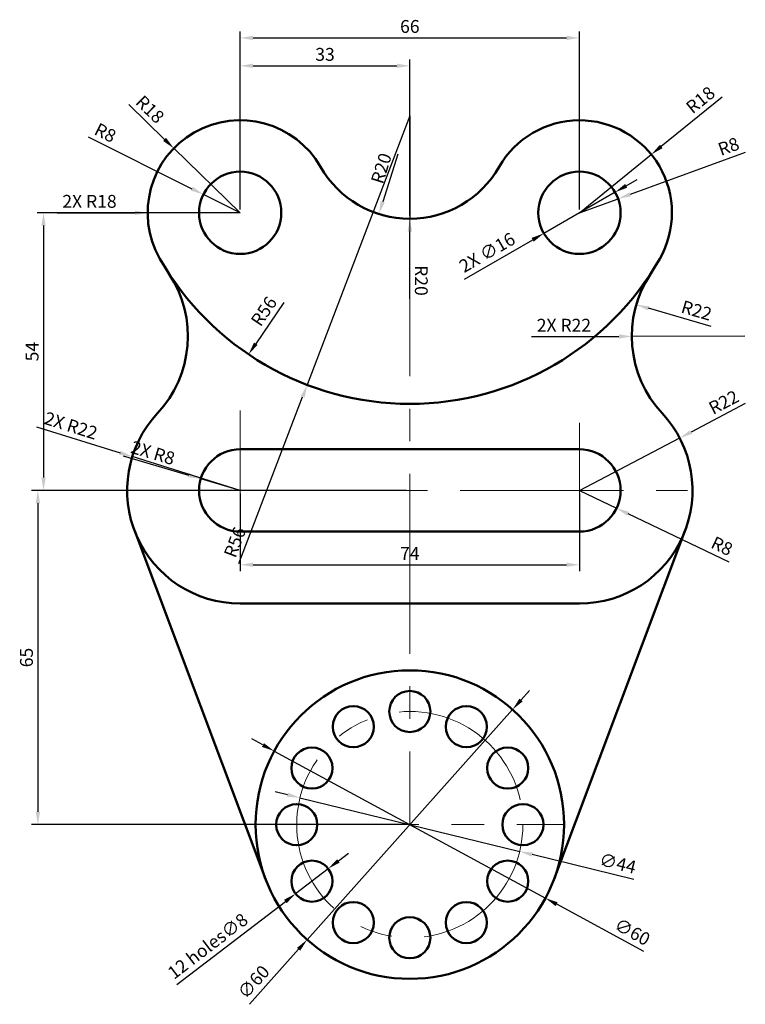
# Model space of a CAD drawing. Units: millimetres. Extents: x 2956 to 3097, y 1555 to 1747.
import ezdxf

# ---------------------------------------------------------------- set-up
doc = ezdxf.new("R2010")
doc.units = ezdxf.units.MM
doc.linetypes.add('CENTER', pattern=[50.8, 31.75, -6.35, 6.35, -6.35])
for name, color, linetype, lineweight in [('M-CNTR', 4, 'CENTER', 18), ('M-DIMS', 2, 'Continuous', 25), ('M-OUTL', 7, 'Continuous', 50)]:
    doc.layers.add(name, color=color, linetype=linetype, lineweight=lineweight)
doc.styles.get("Standard").update_dxf_attribs({"font": 'arial.ttf'})
doc.dimstyles.new('ISO-25', dxfattribs={"dimtxt": 2.5, "dimasz": 2.5, "dimexe": 1.25, "dimexo": 0.625, "dimtad": 1, "dimtxsty": 'Standard', "dimcen": 2.5, "dimadec": 0, "dimazin": 0, "dimtfac": 1, "dimtmove": 0, "dimatfit": 3, "dimfxl": 1, "dimarcsym": 0})

# ---------------------------------------------------------------- blocks, each defined once
blk = doc.blocks.new('*U2')
blk.add_circle((0, 0), 4)
blk = doc.blocks.new('*U3')
at = {"layer": 'M-OUTL', "color": 0, "linetype": 'ByBlock', "lineweight": -2, "transparency": 16777216}
for p, rotation in [((3020.97, 1609.09), 30), ((3042.97, 1609.09), 330), ((3012.92, 1601.04), 59.99999999999999), ((3051.02, 1601.04), 300), ((3009.97, 1590.04), 90), ((3053.97, 1590.04), 269.9999999999999), ((3012.92, 1579.04), 120), ((3051.02, 1579.04), 240), ((3020.97, 1570.99), 150), ((3042.97, 1570.99), 210), ((3031.97, 1568.04), 180)]:
    blk.add_blockref('*U2', p, dxfattribs=dict(at, rotation=rotation))
blk.add_blockref('*U2', (3031.97, 1612.04), dxfattribs=at)
blk = doc.blocks.new('*D4')
at = {"layer": 'Defpoints', "color": 0, "lineweight": -3, "transparency": 16777216}
for p in [(3064.97, 1743.06), (2998.97, 1709.04), (3064.97, 1709.04)]:
    blk.add_point(p, dxfattribs=at)
at = {"layer": 'M-DIMS', "color": 0, "lineweight": -2, "transparency": 16777216}
for p, q in [((2998.97, 1709.67), (2998.97, 1744.31)), ((3001.47, 1743.06), (3062.47, 1743.06)), ((3064.97, 1709.67), (3064.97, 1744.31))]:
    blk.add_line(p, q, dxfattribs=at)
at = {"layer": 'M-DIMS', "color": 0, "lineweight": -3, "transparency": 16777216}
for points in [[(3001.47, 1743.47), (3001.47, 1742.64), (2998.97, 1743.06)], [(3062.47, 1743.47), (3062.47, 1742.64), (3064.97, 1743.06)]]:
    blk.add_solid(points, dxfattribs=at)
at = {"layer": 'M-DIMS', "color": 0, "transparency": 16777216, "insert": (3031.97, 1744.96), "char_height": 2.5, "attachment_point": 5}
blk.add_mtext('66', dxfattribs=at)
blk = doc.blocks.new('*D5')
at = {"layer": 'Defpoints', "color": 0, "lineweight": -3, "transparency": 16777216}
for p in [(3078.95, 1720.38), (3064.97, 1709.04)]:
    blk.add_point(p, dxfattribs=at)
at = {"layer": 'M-DIMS', "color": 0, "lineweight": -2, "transparency": 16777216}
for p, q in [((3092.72, 1731.55), (3080.89, 1721.96)), ((3064.97, 1709.04), (3078.95, 1720.38))]:
    blk.add_line(p, q, dxfattribs=at)
at = {"layer": 'M-DIMS', "color": 0, "lineweight": -3, "transparency": 16777216}
blk.add_solid([(3080.63, 1722.28), (3081.15, 1721.63), (3078.95, 1720.38)], dxfattribs=at)
at = {"layer": 'M-DIMS', "color": 0, "transparency": 16777216, "insert": (3088.71, 1730.75), "char_height": 2.5, "attachment_point": 5, "rotation": 39.0521}
blk.add_mtext('R18', dxfattribs=at)
blk = doc.blocks.new('*D6')
at = {"layer": 'Defpoints', "color": 0, "lineweight": -3, "transparency": 16777216}
for p in [(3072.49, 1711.77), (3064.97, 1709.04)]:
    blk.add_point(p, dxfattribs=at)
at = {"layer": 'M-DIMS', "color": 0, "lineweight": -2, "transparency": 16777216}
for p, q in [((3097.22, 1720.76), (3074.84, 1712.63)), ((3064.97, 1709.04), (3072.49, 1711.77))]:
    blk.add_line(p, q, dxfattribs=at)
at = {"layer": 'M-DIMS', "color": 0, "lineweight": -3, "transparency": 16777216}
blk.add_solid([(3074.7, 1713.02), (3074.98, 1712.24), (3072.49, 1711.77)], dxfattribs=at)
at = {"layer": 'M-DIMS', "color": 0, "transparency": 16777216, "insert": (3094.09, 1721.65), "char_height": 2.5, "attachment_point": 5, "rotation": 19.9709}
blk.add_mtext('R8', dxfattribs=at)
blk = doc.blocks.new('*D7')
at = {"layer": 'Defpoints', "color": 0, "lineweight": -3, "transparency": 16777216}
for p in [(2991.81, 1712.61), (2998.97, 1709.04)]:
    blk.add_point(p, dxfattribs=at)
at = {"layer": 'M-DIMS', "color": 0, "lineweight": -2, "transparency": 16777216}
for p, q in [((2969.38, 1723.79), (2989.57, 1713.73)), ((2998.97, 1709.04), (2991.81, 1712.61))]:
    blk.add_line(p, q, dxfattribs=at)
at = {"layer": 'M-DIMS', "color": 0, "lineweight": -3, "transparency": 16777216}
blk.add_solid([(2989.76, 1714.1), (2989.39, 1713.35), (2991.81, 1712.61)], dxfattribs=at)
at = {"layer": 'M-DIMS', "color": 0, "transparency": 16777216, "insert": (2972.59, 1724.32), "char_height": 2.5, "attachment_point": 5, "rotation": 333.5006}
blk.add_mtext('R8', dxfattribs=at)
blk = doc.blocks.new('*D8')
at = {"layer": 'Defpoints', "color": 0, "lineweight": -3, "transparency": 16777216}
for p in [(2986.05, 1721.58), (2998.97, 1709.04)]:
    blk.add_point(p, dxfattribs=at)
at = {"layer": 'M-DIMS', "color": 0, "lineweight": -2, "transparency": 16777216}
for p, q in [((2977.28, 1730.09), (2984.26, 1723.32)), ((2998.97, 1709.04), (2986.05, 1721.58))]:
    blk.add_line(p, q, dxfattribs=at)
at = {"layer": 'M-DIMS', "color": 0, "lineweight": -3, "transparency": 16777216}
blk.add_solid([(2984.55, 1723.62), (2983.97, 1723.02), (2986.05, 1721.58)], dxfattribs=at)
at = {"layer": 'M-DIMS', "color": 0, "transparency": 16777216, "insert": (2981.2, 1728.94), "char_height": 2.5, "attachment_point": 5, "rotation": 315.858}
blk.add_mtext('R18', dxfattribs=at)
blk = doc.blocks.new('*D9')
at = {"layer": 'Defpoints', "color": 0, "lineweight": -3, "transparency": 16777216}
for p in [(2998.97, 1709.04), (2960.71, 1655.04), (2998.97, 1655.04)]:
    blk.add_point(p, dxfattribs=at)
at = {"layer": 'M-DIMS', "color": 0, "lineweight": -2, "transparency": 16777216}
for p, q in [((2998.34, 1709.04), (2959.46, 1709.04)), ((2960.71, 1706.54), (2960.71, 1657.54)), ((2998.34, 1655.04), (2959.46, 1655.04))]:
    blk.add_line(p, q, dxfattribs=at)
at = {"layer": 'M-DIMS', "color": 0, "lineweight": -3, "transparency": 16777216}
for points in [[(2960.29, 1706.54), (2961.12, 1706.54), (2960.71, 1709.04)], [(2960.29, 1657.54), (2961.12, 1657.54), (2960.71, 1655.04)]]:
    blk.add_solid(points, dxfattribs=at)
at = {"layer": 'M-DIMS', "color": 0, "transparency": 16777216, "insert": (2958.81, 1682.04), "char_height": 2.5, "attachment_point": 5, "rotation": 90}
blk.add_mtext('54', dxfattribs=at)
blk = doc.blocks.new('*D10')
at = {"layer": 'Defpoints', "color": 0, "lineweight": -3, "transparency": 16777216}
for p in [(3031.97, 1727.88), (3000.59, 1681.5)]:
    blk.add_point(p, dxfattribs=at)
at = {"layer": 'M-DIMS', "color": 0, "lineweight": -2, "transparency": 16777216}
blk.add_line((3007.44, 1691.62), (3001.99, 1683.57), dxfattribs=at)
at = {"layer": 'M-DIMS', "color": 0, "lineweight": -3, "transparency": 16777216}
blk.add_solid([(3001.65, 1683.8), (3002.34, 1683.34), (3000.59, 1681.5)], dxfattribs=at)
at = {"layer": 'M-DIMS', "color": 0, "transparency": 16777216, "insert": (3003.84, 1689.7), "char_height": 2.5, "attachment_point": 5, "rotation": 55.9212}
blk.add_mtext('R56', dxfattribs=at)
blk = doc.blocks.new('*D11')
at = {"layer": 'Defpoints', "color": 0, "lineweight": -3, "transparency": 16777216}
for p in [(3076.02, 1691.15), (3097.15, 1685.04)]:
    blk.add_point(p, dxfattribs=at)
at = {"layer": 'M-DIMS', "color": 0, "lineweight": -2, "transparency": 16777216}
blk.add_line((3090.61, 1686.93), (3078.42, 1690.46), dxfattribs=at)
at = {"layer": 'M-DIMS', "color": 0, "lineweight": -3, "transparency": 16777216}
blk.add_solid([(3078.54, 1690.86), (3078.3, 1690.06), (3076.02, 1691.15)], dxfattribs=at)
at = {"layer": 'M-DIMS', "color": 0, "transparency": 16777216, "insert": (3087.67, 1689.74), "char_height": 2.5, "attachment_point": 5, "rotation": 343.8873}
blk.add_mtext('R22', dxfattribs=at)
blk = doc.blocks.new('*D12')
at = {"layer": 'Defpoints', "color": 0, "lineweight": -3, "transparency": 16777216}
for p in [(3084.47, 1665.24), (3064.97, 1655.04)]:
    blk.add_point(p, dxfattribs=at)
at = {"layer": 'M-DIMS', "color": 0, "lineweight": -2, "transparency": 16777216}
for p, q in [((3097.24, 1671.92), (3086.68, 1666.39)), ((3064.97, 1655.04), (3084.47, 1665.24))]:
    blk.add_line(p, q, dxfattribs=at)
at = {"layer": 'M-DIMS', "color": 0, "lineweight": -3, "transparency": 16777216}
blk.add_solid([(3086.49, 1666.76), (3086.87, 1666.03), (3084.47, 1665.24)], dxfattribs=at)
at = {"layer": 'M-DIMS', "color": 0, "transparency": 16777216, "insert": (3093.18, 1671.91), "char_height": 2.5, "attachment_point": 5, "rotation": 27.6065}
blk.add_mtext('R22', dxfattribs=at)
blk = doc.blocks.new('*D13')
at = {"layer": 'Defpoints', "color": 0, "lineweight": -3, "transparency": 16777216}
for p in [(2998.97, 1655.04), (3064.97, 1655.04), (3064.97, 1640.58)]:
    blk.add_point(p, dxfattribs=at)
at = {"layer": 'M-DIMS', "color": 0, "lineweight": -2, "transparency": 16777216}
for p, q in [((2998.97, 1654.42), (2998.97, 1639.33)), ((3064.97, 1654.42), (3064.97, 1639.33)), ((3001.47, 1640.58), (3062.47, 1640.58))]:
    blk.add_line(p, q, dxfattribs=at)
at = {"layer": 'M-DIMS', "color": 0, "lineweight": -3, "transparency": 16777216}
for points in [[(3001.47, 1641), (3001.47, 1640.17), (2998.97, 1640.58)], [(3062.47, 1641), (3062.47, 1640.17), (3064.97, 1640.58)]]:
    blk.add_solid(points, dxfattribs=at)
at = {"layer": 'M-DIMS', "color": 0, "transparency": 16777216, "insert": (3031.97, 1642.46), "char_height": 2.5, "attachment_point": 5}
blk.add_mtext('74', dxfattribs=at)
blk = doc.blocks.new('*D14')
at = {"layer": 'Defpoints', "color": 0, "lineweight": -3, "transparency": 16777216}
for p in [(3064.97, 1655.04), (3072.18, 1651.59)]:
    blk.add_point(p, dxfattribs=at)
at = {"layer": 'M-DIMS', "color": 0, "lineweight": -2, "transparency": 16777216}
for p, q in [((3064.97, 1655.04), (3072.18, 1651.59)), ((3094.12, 1641.08), (3074.44, 1650.51))]:
    blk.add_line(p, q, dxfattribs=at)
at = {"layer": 'M-DIMS', "color": 0, "lineweight": -3, "transparency": 16777216}
blk.add_solid([(3074.62, 1650.88), (3074.26, 1650.13), (3072.18, 1651.59)], dxfattribs=at)
at = {"layer": 'M-DIMS', "color": 0, "transparency": 16777216, "insert": (3092.56, 1643.94), "char_height": 2.5, "attachment_point": 5, "rotation": 334.407}
blk.add_mtext('R8', dxfattribs=at)
blk = doc.blocks.new('*D15')
at = {"layer": 'Defpoints', "color": 0, "lineweight": -3, "transparency": 16777216}
for p in [(3031.97, 1655.04), (2959.61, 1590.04), (3031.97, 1590.04)]:
    blk.add_point(p, dxfattribs=at)
at = {"layer": 'M-DIMS', "color": 0, "lineweight": -2, "transparency": 16777216}
for p, q in [((3031.34, 1655.04), (2958.36, 1655.04)), ((2959.61, 1652.54), (2959.61, 1592.54)), ((3031.34, 1590.04), (2958.36, 1590.04))]:
    blk.add_line(p, q, dxfattribs=at)
at = {"layer": 'M-DIMS', "color": 0, "lineweight": -3, "transparency": 16777216}
for points in [[(2959.19, 1652.54), (2960.03, 1652.54), (2959.61, 1655.04)], [(2959.19, 1592.54), (2960.03, 1592.54), (2959.61, 1590.04)]]:
    blk.add_solid(points, dxfattribs=at)
at = {"layer": 'M-DIMS', "color": 0, "transparency": 16777216, "insert": (2957.71, 1622.54), "char_height": 2.5, "attachment_point": 5, "rotation": 90}
blk.add_mtext('65', dxfattribs=at)
blk = doc.blocks.new('*D16')
at = {"layer": 'Defpoints', "color": 0, "lineweight": -3, "transparency": 16777216}
for p in [(3031.97, 1727.88), (3025.95, 1708.81)]:
    blk.add_point(p, dxfattribs=at)
at = {"layer": 'M-DIMS', "color": 0, "lineweight": -2, "transparency": 16777216}
blk.add_line((3029.62, 1720.46), (3026.7, 1711.2), dxfattribs=at)
at = {"layer": 'M-DIMS', "color": 0, "lineweight": -3, "transparency": 16777216}
blk.add_solid([(3026.3, 1711.32), (3027.1, 1711.07), (3025.95, 1708.81)], dxfattribs=at)
at = {"layer": 'M-DIMS', "color": 0, "transparency": 16777216, "insert": (3026.72, 1717.59), "char_height": 2.5, "attachment_point": 5, "rotation": 72.4688}
blk.add_mtext('R20', dxfattribs=at)
blk = doc.blocks.new('*D17')
at = {"layer": 'Defpoints', "color": 0, "lineweight": -3, "transparency": 16777216}
for p in [(3010.6, 1595.26), (3053.34, 1584.82)]:
    blk.add_point(p, dxfattribs=at)
at = {"layer": 'M-DIMS', "color": 0, "lineweight": -2, "transparency": 16777216}
for p, q in [((3008.17, 1595.86), (3005.74, 1596.45)), ((3010.6, 1595.26), (3053.34, 1584.82)), ((3075.55, 1579.39), (3055.77, 1584.23))]:
    blk.add_line(p, q, dxfattribs=at)
at = {"layer": 'M-DIMS', "color": 0, "lineweight": -3, "transparency": 16777216}
for points in [[(3008.27, 1596.26), (3008.07, 1595.45), (3010.6, 1595.26)], [(3055.87, 1584.63), (3055.67, 1583.82), (3053.34, 1584.82)]]:
    blk.add_solid(points, dxfattribs=at)
at = {"layer": 'M-DIMS', "color": 0, "transparency": 16777216, "insert": (3072.35, 1582.2), "char_height": 2.5, "attachment_point": 5, "rotation": 346.271}
blk.add_mtext('∅44', dxfattribs=at)
blk = doc.blocks.new('*D18')
at = {"layer": 'Defpoints', "color": 0, "lineweight": -3, "transparency": 16777216}
for p in [(3051.95, 1612.42), (3011.99, 1567.66)]:
    blk.add_point(p, dxfattribs=at)
at = {"layer": 'M-DIMS', "color": 0, "lineweight": -2, "transparency": 16777216}
for p, q in [((3053.61, 1614.29), (3055.28, 1616.15)), ((3051.95, 1612.42), (3011.99, 1567.66)), ((3000.77, 1555.09), (3010.33, 1565.8))]:
    blk.add_line(p, q, dxfattribs=at)
at = {"layer": 'M-DIMS', "color": 0, "lineweight": -3, "transparency": 16777216}
for points in [[(3053.3, 1614.56), (3053.92, 1614.01), (3051.95, 1612.42)], [(3010.02, 1566.07), (3010.64, 1565.52), (3011.99, 1567.66)]]:
    blk.add_solid(points, dxfattribs=at)
at = {"layer": 'M-DIMS', "color": 0, "transparency": 16777216, "insert": (3001.81, 1559.22), "char_height": 2.5, "attachment_point": 5, "rotation": 48.2455}
blk.add_mtext('∅60', dxfattribs=at)
blk = doc.blocks.new('*D19')
at = {"layer": 'Defpoints', "color": 0, "lineweight": -3, "transparency": 16777216}
for p in [(3016.09, 1581.47), (3009.74, 1576.61)]:
    blk.add_point(p, dxfattribs=at)
at = {"layer": 'M-DIMS', "color": 0, "lineweight": -2, "transparency": 16777216}
for p, q in [((3018.08, 1582.99), (3020.06, 1584.51)), ((3016.09, 1581.47), (3009.74, 1576.61)), ((2986.67, 1558.95), (3007.76, 1575.09))]:
    blk.add_line(p, q, dxfattribs=at)
at = {"layer": 'M-DIMS', "color": 0, "lineweight": -3, "transparency": 16777216}
for points in [[(3017.83, 1583.32), (3018.33, 1582.66), (3016.09, 1581.47)], [(3007.5, 1575.42), (3008.01, 1574.76), (3009.74, 1576.61)]]:
    blk.add_solid(points, dxfattribs=at)
at = {"layer": 'M-DIMS', "color": 0, "transparency": 16777216, "insert": (2992.85, 1566.16), "char_height": 2.5, "attachment_point": 5, "rotation": 37.4262}
blk.add_mtext('12 holes∅8', dxfattribs=at)
blk = doc.blocks.new('HOLE-D16')
blk.add_circle((8, 8), 8)
blk = doc.blocks.new('*D21')
at = {"layer": 'Defpoints', "color": 0, "lineweight": -3, "transparency": 16777216}
for p in [(3031.97, 1737.63), (2998.97, 1709.04), (3031.97, 1707.88)]:
    blk.add_point(p, dxfattribs=at)
at = {"layer": 'M-DIMS', "color": 0, "lineweight": -2, "transparency": 16777216}
for p, q in [((2998.97, 1709.67), (2998.97, 1738.88)), ((3001.47, 1737.63), (3029.47, 1737.63)), ((3031.97, 1708.51), (3031.97, 1738.88))]:
    blk.add_line(p, q, dxfattribs=at)
at = {"layer": 'M-DIMS', "color": 0, "lineweight": -3, "transparency": 16777216}
for points in [[(3001.47, 1738.05), (3001.47, 1737.22), (2998.97, 1737.63)], [(3029.47, 1738.05), (3029.47, 1737.22), (3031.97, 1737.63)]]:
    blk.add_solid(points, dxfattribs=at)
at = {"layer": 'M-DIMS', "color": 0, "transparency": 16777216, "insert": (3015.47, 1739.53), "char_height": 2.5, "attachment_point": 5}
blk.add_mtext('33', dxfattribs=at)
blk = doc.blocks.new('*D22')
at = {"layer": 'Defpoints', "color": 0, "lineweight": -3, "transparency": 16777216}
for p in [(3071.9, 1713.04), (3058.04, 1705.04)]:
    blk.add_point(p, dxfattribs=at)
at = {"layer": 'M-DIMS', "color": 0, "lineweight": -2, "transparency": 16777216}
for p, q in [((3074.06, 1714.29), (3076.23, 1715.54)), ((3071.9, 1713.04), (3058.04, 1705.04)), ((3042.6, 1696.13), (3055.88, 1703.79))]:
    blk.add_line(p, q, dxfattribs=at)
at = {"layer": 'M-DIMS', "color": 0, "lineweight": -3, "transparency": 16777216}
for points in [[(3073.85, 1714.65), (3074.27, 1713.93), (3071.9, 1713.04)], [(3055.67, 1704.15), (3056.08, 1703.43), (3058.04, 1705.04)]]:
    blk.add_solid(points, dxfattribs=at)
at = {"layer": 'M-DIMS', "color": 0, "transparency": 16777216, "insert": (3047.17, 1701.04), "char_height": 2.5, "attachment_point": 5, "rotation": 30.0016}
blk.add_mtext('2X ∅16', dxfattribs=at)
blk = doc.blocks.new('*D23')
at = {"layer": 'Defpoints', "color": 0, "lineweight": -3, "transparency": 16777216}
for p in [(2980.97, 1709.04), (2998.97, 1709.04)]:
    blk.add_point(p, dxfattribs=at)
at = {"layer": 'M-DIMS', "color": 0, "lineweight": -2, "transparency": 16777216}
for p, q in [((2963.33, 1709.04), (2978.47, 1709.04)), ((2998.97, 1709.04), (2980.97, 1709.04))]:
    blk.add_line(p, q, dxfattribs=at)
at = {"layer": 'M-DIMS', "color": 0, "lineweight": -3, "transparency": 16777216}
blk.add_solid([(2978.47, 1709.46), (2978.47, 1708.62), (2980.97, 1709.04)], dxfattribs=at)
at = {"layer": 'M-DIMS', "color": 0, "transparency": 16777216, "insert": (2969.65, 1710.94), "char_height": 2.5, "attachment_point": 5, "rotation": 0.0005}
blk.add_mtext('2X R18', dxfattribs=at)
blk = doc.blocks.new('*D24')
at = {"layer": 'Defpoints', "color": 0, "lineweight": -3, "transparency": 16777216}
for p in [(3031.97, 1727.88), (3031.97, 1707.88)]:
    blk.add_point(p, dxfattribs=at)
at = {"layer": 'M-DIMS', "color": 0, "lineweight": -2, "transparency": 16777216}
for p, q in [((3031.97, 1727.88), (3031.97, 1707.88)), ((3031.97, 1692.28), (3031.97, 1705.38))]:
    blk.add_line(p, q, dxfattribs=at)
at = {"layer": 'M-DIMS', "color": 0, "lineweight": -3, "transparency": 16777216}
blk.add_solid([(3032.39, 1705.38), (3031.55, 1705.38), (3031.97, 1707.88)], dxfattribs=at)
at = {"layer": 'M-DIMS', "color": 0, "transparency": 16777216, "insert": (3033.87, 1695.88), "char_height": 2.5, "attachment_point": 5, "rotation": 270.0006}
blk.add_mtext('R20', dxfattribs=at)
blk = doc.blocks.new('*D25')
at = {"layer": 'Defpoints', "color": 0, "lineweight": -3, "transparency": 16777216}
for p in [(3031.97, 1727.88), (3012, 1675.56)]:
    blk.add_point(p, dxfattribs=at)
at = {"layer": 'M-DIMS', "color": 0, "lineweight": -2, "transparency": 16777216}
for p, q in [((3031.97, 1727.88), (3012, 1675.56)), ((2998.73, 1640.8), (3011.11, 1673.23))]:
    blk.add_line(p, q, dxfattribs=at)
at = {"layer": 'M-DIMS', "color": 0, "lineweight": -3, "transparency": 16777216}
blk.add_solid([(3010.72, 1673.38), (3011.5, 1673.08), (3012, 1675.56)], dxfattribs=at)
at = {"layer": 'M-DIMS', "color": 0, "transparency": 16777216, "insert": (2998.24, 1644.85), "char_height": 2.5, "attachment_point": 5, "rotation": 69.1098}
blk.add_mtext('R56', dxfattribs=at)
blk = doc.blocks.new('*D26')
at = {"layer": 'Defpoints', "color": 0, "lineweight": -3, "transparency": 16777216}
for p in [(3075.15, 1685), (3097.15, 1685.04)]:
    blk.add_point(p, dxfattribs=at)
at = {"layer": 'M-DIMS', "color": 0, "lineweight": -2, "transparency": 16777216}
for p, q in [((3055.65, 1684.96), (3072.65, 1685)), ((3097.15, 1685.04), (3075.15, 1685))]:
    blk.add_line(p, q, dxfattribs=at)
at = {"layer": 'M-DIMS', "color": 0, "lineweight": -3, "transparency": 16777216}
blk.add_solid([(3072.65, 1685.41), (3072.65, 1684.58), (3075.15, 1685)], dxfattribs=at)
at = {"layer": 'M-DIMS', "color": 0, "transparency": 16777216, "insert": (3061.95, 1686.85), "char_height": 2.5, "attachment_point": 5, "rotation": 0.1161}
blk.add_mtext('2X R22', dxfattribs=at)
blk = doc.blocks.new('*D27')
at = {"layer": 'Defpoints', "color": 0, "lineweight": -3, "transparency": 16777216}
for p in [(2977.97, 1661.61), (2998.97, 1655.04)]:
    blk.add_point(p, dxfattribs=at)
at = {"layer": 'M-DIMS', "color": 0, "lineweight": -2, "transparency": 16777216}
for p, q in [((2959.36, 1667.43), (2975.59, 1662.35)), ((2998.97, 1655.04), (2977.97, 1661.61))]:
    blk.add_line(p, q, dxfattribs=at)
at = {"layer": 'M-DIMS', "color": 0, "lineweight": -3, "transparency": 16777216}
blk.add_solid([(2975.71, 1662.75), (2975.46, 1661.96), (2977.97, 1661.61)], dxfattribs=at)
at = {"layer": 'M-DIMS', "color": 0, "transparency": 16777216, "insert": (2965.94, 1667.34), "char_height": 2.5, "attachment_point": 5, "rotation": 342.6316}
blk.add_mtext('2X R22', dxfattribs=at)
blk = doc.blocks.new('*D28')
at = {"layer": 'Defpoints', "color": 0, "lineweight": -3, "transparency": 16777216}
for p in [(2991.3, 1657.3), (2998.97, 1655.04)]:
    blk.add_point(p, dxfattribs=at)
at = {"layer": 'M-DIMS', "color": 0, "lineweight": -2, "transparency": 16777216}
for p, q in [((2976.23, 1661.74), (2988.9, 1658.01)), ((2998.97, 1655.04), (2991.3, 1657.3))]:
    blk.add_line(p, q, dxfattribs=at)
at = {"layer": 'M-DIMS', "color": 0, "lineweight": -3, "transparency": 16777216}
blk.add_solid([(2989.02, 1658.41), (2988.78, 1657.61), (2991.3, 1657.3)], dxfattribs=at)
at = {"layer": 'M-DIMS', "color": 0, "transparency": 16777216, "insert": (2981.9, 1662.05), "char_height": 2.5, "attachment_point": 5, "rotation": 343.5897}
blk.add_mtext('2X R8', dxfattribs=at)
blk = doc.blocks.new('*D29')
at = {"layer": 'Defpoints', "color": 0, "lineweight": -3, "transparency": 16777216}
for p in [(3005.59, 1604.34), (3058.35, 1575.75)]:
    blk.add_point(p, dxfattribs=at)
at = {"layer": 'M-DIMS', "color": 0, "lineweight": -2, "transparency": 16777216}
for p, q in [((3003.4, 1605.53), (3001.2, 1606.72)), ((3005.59, 1604.34), (3058.35, 1575.75)), ((3077.49, 1565.37), (3060.54, 1574.56))]:
    blk.add_line(p, q, dxfattribs=at)
at = {"layer": 'M-DIMS', "color": 0, "lineweight": -3, "transparency": 16777216}
for points in [[(3003.59, 1605.89), (3003.2, 1605.16), (3005.59, 1604.34)], [(3060.74, 1574.92), (3060.34, 1574.19), (3058.35, 1575.75)]]:
    blk.add_solid(points, dxfattribs=at)
at = {"layer": 'M-DIMS', "color": 0, "transparency": 16777216, "insert": (3075.11, 1568.9), "char_height": 2.5, "attachment_point": 5, "rotation": 331.5437}
blk.add_mtext('∅60', dxfattribs=at)

msp = doc.modelspace()

# ---------------------------------------------------------------- linework, layer by layer
at = {"layer": 'M-CNTR'}
for p, q in [((3031.97, 1709.041), (3031.97, 1727.883)), ((3031.97, 1709.041), (3031.97, 1655.041)), ((2998.97, 1647.041), (2998.97, 1670.608)), ((3064.97, 1663.041), (3064.97, 1668.157)), ((3064.97, 1663.041), (3064.97, 1640.582)), ((2990.97, 1655.041), (2967.716, 1655.041)), ((2990.97, 1655.041), (3085.99, 1655.041)), ((3031.97, 1655.041), (3031.97, 1590.041)), ((2998.97, 1647.041), (2998.97, 1640.296)), ((3001.97, 1590.041), (2963.392, 1590.041)), ((3001.97, 1590.041), (3061.97, 1590.041))]:
    msp.add_line(p, q, dxfattribs=at)
msp.add_circle((3031.97, 1590.041), 22, dxfattribs=at)
at = {"layer": 'M-OUTL'}
for p, q in [((2998.97, 1663.041), (3064.97, 1663.041)), ((2978.379, 1647.295), (3003.891, 1579.478)), ((2998.97, 1647.041), (3064.97, 1647.041)), ((3060.049, 1579.478), (3085.561, 1647.295)), ((2998.97, 1633.041), (3064.97, 1633.041))]:
    msp.add_line(p, q, dxfattribs=at)
msp.add_circle((3031.97, 1590.041), 30, dxfattribs=at)
for centre, radius, start, end in [((2998.97, 1709.041), 18, 29.72433, 209.72433), ((3064.97, 1709.041), 18, 330.27567, 150.27567), ((3031.97, 1727.883), 20, 209.72433, 330.27567), ((3031.97, 1727.883), 56, 209.72433, 213.31244), ((3031.97, 1727.883), 56, 209.72433, 330.27567), ((3031.97, 1727.883), 56, 326.68756, 330.27567), ((2966.786, 1685.045), 22, 317.00786, 33.31244), ((3097.153, 1685.045), 22, 146.68756, 222.99214), ((2998.97, 1655.041), 22, 137.00786, 270), ((3064.97, 1655.041), 22, 270, 42.99214), ((2998.97, 1655.041), 8, 90, 270), ((3064.97, 1655.041), 8, 270, 90)]:
    msp.add_arc(centre, radius, start, end, dxfattribs=at)

# ---------------------------------------------------------------- block references
for name, p in [('HOLE-D16', (2990.97, 1701.041)), ('HOLE-D16', (3056.97, 1701.041)), ('*U3', (0, 0))]:
    msp.add_blockref(name, p, dxfattribs=at)

# ---------------------------------------------------------------- dimensions: what is measured, and where the dimension line sits
at = {"layer": 'M-DIMS'}
for base, p2, override, picture, middle in [((3064.97, 1743.057), (3064.97, 1709.041), {"dimclrd": 0, "dimclre": 0, "dimclrt": 0}, '*D4', (3031.97, 1744.959)), ((3031.97, 1737.633), (3031.97, 1707.883), {"dimdec": 0, "dimlfac": 1, "dimrnd": 0, "dimzin": 0, "dimdsep": 46, "dimlunit": 2}, '*D21', (3015.47, 1739.535))]:
    dim = msp.add_linear_dim(base=base, p1=(2998.97, 1709.041), p2=p2, dimstyle='ISO-25', override=override, dxfattribs=at)
    dim.commit()
    dim.dimension.update_dxf_attribs({"geometry": picture, "text_midpoint": middle})
for center, mpoint, override, picture, middle in [((3064.97, 1709.041), (3078.948, 1720.382), {"dimclrd": 0, "dimclre": 0, "dimclrt": 0}, '*D5', (3089.912, 1729.276)), ((3031.97, 1727.883), (3012.001, 1675.564), {"dimdec": 0, "dimlfac": 1, "dimrnd": 0, "dimzin": 0, "dimdsep": 46, "dimlunit": 2}, '*D25', (3000.02, 1644.172)), ((3031.97, 1727.883), (3000.591, 1681.5), {"dimclrd": 0, "dimclre": 0, "dimclrt": 0}, '*D10', (3005.416, 1688.632)), ((3031.97, 1727.883), (3025.945, 1708.812), {"dimclrd": 0, "dimclre": 0, "dimclrt": 0}, '*D16', (3028.538, 1717.019)), ((3031.97, 1727.883), (3031.97, 1707.883), {"dimdec": 0, "dimlfac": 1, "dimrnd": 0, "dimzin": 0, "dimdsep": 46, "dimlunit": 2}, '*D24', (3031.97, 1695.883)), ((2998.97, 1709.041), (2991.81, 1712.611), {"dimclrd": 0, "dimclre": 0, "dimclrt": 0}, '*D7', (2971.743, 1722.616)), ((3064.97, 1709.041), (3072.489, 1711.774), {"dimclrd": 0, "dimclre": 0, "dimclrt": 0}, '*D6', (3094.74, 1719.859)), ((3097.153, 1685.045), (3076.018, 1691.15), {"dimclrd": 0, "dimclre": 0, "dimclrt": 0}, '*D11', (3087.153, 1687.934)), ((3064.97, 1655.041), (3084.465, 1665.236), {"dimclrd": 0, "dimclre": 0, "dimclrt": 0}, '*D12', (3094.05, 1670.248)), ((3064.97, 1655.041), (3072.185, 1651.585), {"dimclrd": 0, "dimclre": 0, "dimclrt": 0}, '*D14', (3091.735, 1642.221))]:
    dim = msp.add_radius_dim(center=center, mpoint=mpoint, dimstyle='ISO-25', override=override, dxfattribs=at)
    dim.commit()
    dim.dimension.update_dxf_attribs({"geometry": picture, "text_midpoint": middle, "dimtype": 164})
dim = msp.add_radius_dim(center=(2998.97, 1709.041), mpoint=(2986.053, 1721.577), dimstyle='ISO-25', override={"dimclrd": 0, "dimclre": 0, "dimclrt": 0}, dxfattribs=at)
dim.commit()
dim.dimension.update_dxf_attribs({"geometry": '*D8', "text_midpoint": (2981.195, 1728.941)})
for center, mpoint, picture, middle in [((2998.97, 1709.041), (2980.97, 1709.041), '*D23', (2969.648, 1710.942)), ((2998.97, 1655.041), (2991.296, 1657.301), '*D28', (2981.904, 1662.049))]:
    dim = msp.add_radius_dim(center=center, mpoint=mpoint, text='2X <>', dimstyle='ISO-25', override={"dimdec": 0, "dimlfac": 1, "dimrnd": 0, "dimzin": 0, "dimdsep": 46, "dimlunit": 2}, dxfattribs=at)
    dim.commit()
    dim.dimension.update_dxf_attribs({"geometry": picture, "text_midpoint": middle})
dim = msp.add_diameter_dim_2p(p1=(3071.898, 1713.041), p2=(3058.042, 1705.041), text='2X <>', dimstyle='ISO-25', override={"dimdec": 0, "dimlfac": 1, "dimrnd": 0, "dimzin": 0, "dimdsep": 46, "dimlunit": 2}, dxfattribs=at)
dim.commit()
dim.dimension.update_dxf_attribs({"geometry": '*D22', "text_midpoint": (3048.156, 1699.333)})
for base, p1, p2, picture, middle in [((2960.708, 1655.041), (2998.97, 1709.041), (2998.97, 1655.041), '*D9', (2958.811, 1682.041)), ((2959.61, 1590.041), (3031.97, 1655.041), (3031.97, 1590.041), '*D15', (2957.708, 1622.541))]:
    dim = msp.add_linear_dim(base=base, p1=p1, p2=p2, angle=90, dimstyle='ISO-25', override={"dimclrd": 0, "dimclre": 0, "dimclrt": 0}, dxfattribs=at)
    dim.commit()
    dim.dimension.update_dxf_attribs({"geometry": picture, "text_midpoint": middle})
for center, mpoint, picture, middle in [((3097.153, 1685.045), (3075.153, 1685), '*D26', (3061.954, 1684.973)), ((2998.97, 1655.041), (2977.973, 1661.608), '*D27', (2965.375, 1665.549))]:
    dim = msp.add_radius_dim(center=center, mpoint=mpoint, text='2X <>', dimstyle='ISO-25', override={"dimdec": 0, "dimlfac": 1, "dimrnd": 0, "dimzin": 0, "dimdsep": 46, "dimlunit": 2}, dxfattribs=at)
    dim.commit()
    dim.dimension.update_dxf_attribs({"geometry": picture, "text_midpoint": middle, "dimtype": 164})
dim = msp.add_linear_dim(base=(3064.97, 1640.582), p1=(2998.97, 1655.041), p2=(3064.97, 1655.041), text='74', dimstyle='ISO-25', override={"dimclrd": 0, "dimclre": 0, "dimclrt": 0}, dxfattribs=at)
dim.commit()
dim.dimension.update_dxf_attribs({"geometry": '*D13', "text_midpoint": (3031.97, 1642.457)})
for p1, p2, override, picture, middle in [((3051.948, 1612.421), (3011.992, 1567.661), {"dimclrd": 0, "dimclre": 0, "dimclrt": 0}, '*D18', (3003.283, 1557.905)), ((3005.594, 1604.336), (3058.345, 1575.746), {"dimdec": 0, "dimlfac": 1, "dimrnd": 0, "dimzin": 0, "dimdsep": 46, "dimlunit": 2}, '*D29', (3074.17, 1567.17)), ((3010.598, 1595.262), (3053.341, 1584.82), {"dimclrd": 0, "dimclre": 0, "dimclrt": 0}, '*D17', (3071.885, 1580.289))]:
    dim = msp.add_diameter_dim_2p(p1=p1, p2=p2, dimstyle='ISO-25', override=override, dxfattribs=at)
    dim.commit()
    dim.dimension.update_dxf_attribs({"geometry": picture, "text_midpoint": middle, "dimtype": 163})
dim = msp.add_diameter_dim_2p(p1=(3016.094, 1581.472), p2=(3009.741, 1576.61), text='12 holes<>', dimstyle='ISO-25', override={"dimclrd": 0, "dimclre": 0, "dimclrt": 0}, dxfattribs=at)
dim.commit()
dim.dimension.update_dxf_attribs({"geometry": '*D19', "text_midpoint": (2994.044, 1564.598), "dimtype": 163})

doc.saveas('drawing.dxf')
